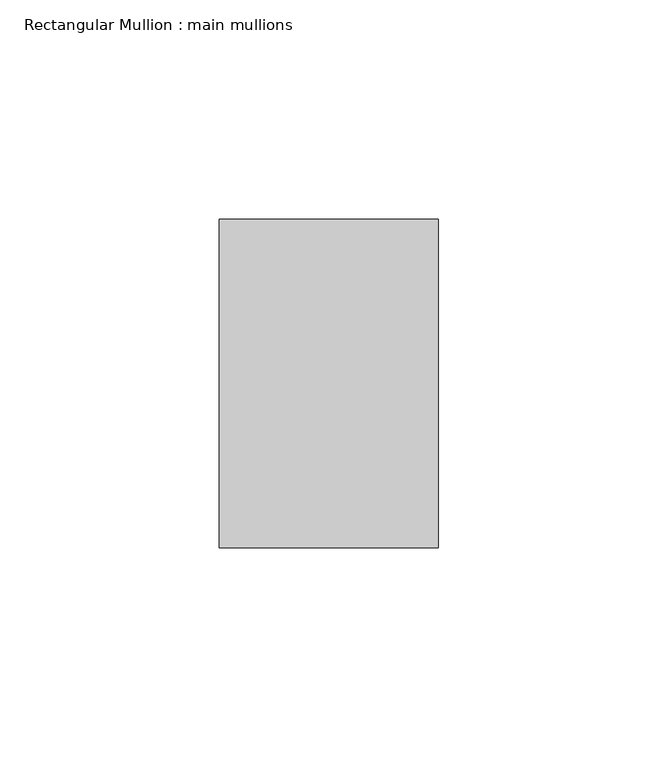
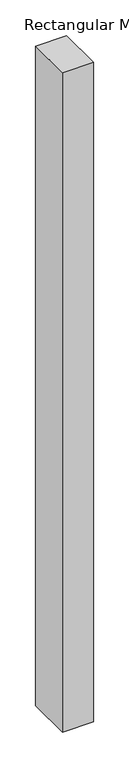
"""IFC4 building model written with IfcOpenShell, lengths in millimetres: member geometry, Rectangular Mullion : main mullions."""

from ifc_helpers import new_model, si_unit, frame, origin, place, context, project, spatial, polyline, outline, extrude, source, transform, mapped, element, save


def rectangular_mullion_main_mullions_8c683149(model_context):
    return source(origin(), model_context, "Body", "SweptSolid", [
        extrude(outline(polyline([(25.0, 37.5), (25.0, -37.5), (-25.0, -37.5), (-25.0, 37.5), (25.0, 37.5)])), frame((0.0, 0.0, -1125.0), z_axis=(0.0, 0.0, 1.0), x_axis=(1.0, 0.0, 0.0)), (0.0, 0.0, 1.0), 1125.0),
    ])


if __name__ == "__main__":
    model = new_model("IFC4")
    model_context = context("Model", 3, world=origin())
    ifc_project = project(units=[si_unit("LENGTHUNIT", "METRE", prefix="MILLI")], contexts=[model_context])
    site = spatial("IfcSite", under=ifc_project)
    building = spatial("IfcBuilding", under=site)
    placement = place(None, origin())
    rectangular_mullion_main_mullions_shape = rectangular_mullion_main_mullions_8c683149(model_context)
    element("IfcMember", 1, ObjectType="Rectangular Mullion : main mullions", at=placement, inside=building, context=model_context, shape_type="MappedRepresentation", body=[
        mapped(rectangular_mullion_main_mullions_shape, transform((0.0, 0.0, 0.0), x_axis=(1.0, 0.0, 0.0), y_axis=(0.0, 1.0, 0.0), z_axis=(0.0, 0.0, 1.0))),
    ])
    save(model, "model.ifc")

# Revit data of these elements
# Type "Rectangular Mullion : main mullions"
#   built-in parameter 1007304 = 0.246063 (stored number, unit not read)
#   built-in parameter 1007301 = 0.082021 (stored number, unit not read)
#   built-in parameter 1007300 = 0.082021 (stored number, unit not read)
# Element 1 (IfcMember, "Rectangular Mullion : main mullions")
#   Materials on its faces: "Aluminum"
# Materials
#   "Aluminum": class "Metal", colour RGB 136 136 136, transparency 0, Description = "Aluminum 6061", Cost = 0
